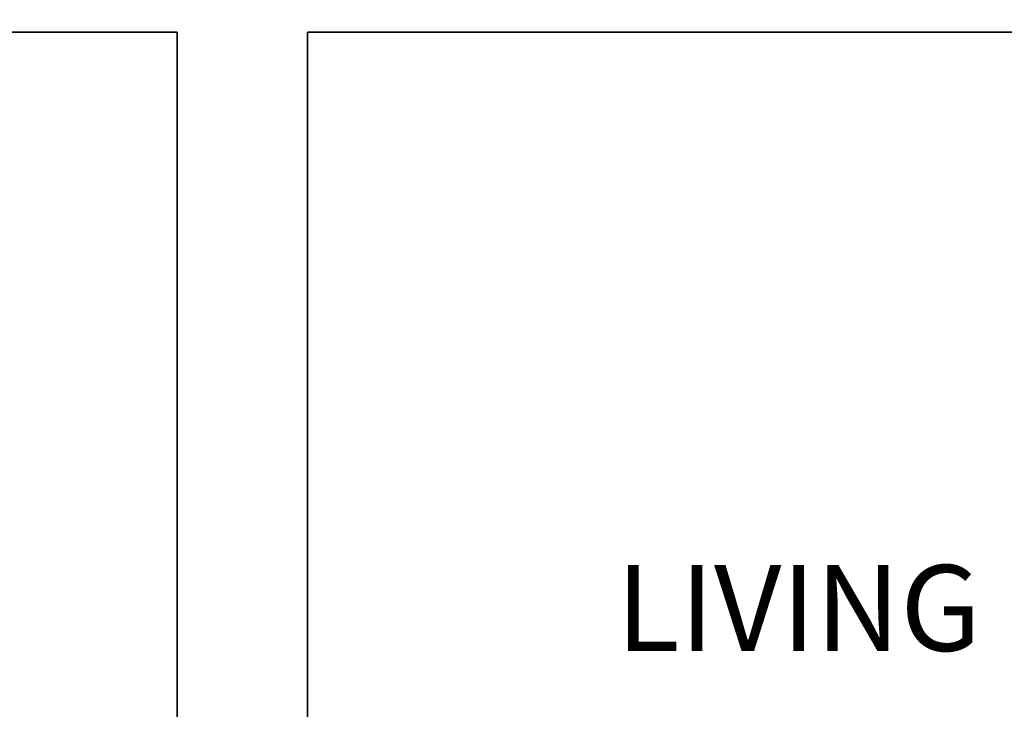
# Model space of a CAD drawing. Units: millimetres. Extents: x 27017497 to 27018854, y 7058029 to 7059154.
# Tile 37 of 91: x 27017621 to 27017689, y 7058386 to 7058433. Entities that reach past the tile are written whole.
import ezdxf

# ---------------------------------------------------------------- set-up
doc = ezdxf.new("R2010")
doc.units = ezdxf.units.MM
for name, color, linetype, lineweight in [('A-ANNO-DIMS', 2, 'Continuous', 18), ('A-AREA-IDEN', 7, 'Continuous', 18), ('A-WALL', 7, 'Continuous', 35)]:
    doc.layers.add(name, color=color, linetype=linetype, lineweight=lineweight)
doc.styles.get("Standard").update_dxf_attribs({"font": 'arial.ttf'})
doc.dimstyles.get("Standard").update_dxf_attribs({"dimtxt": 0.18, "dimasz": 0.18, "dimexe": 0.18, "dimexo": 0.0625, "dimgap": 0.09, "dimtad": 0, "dimtih": 1, "dimtoh": 1, "dimdec": 4, "dimzin": 0, "dimdsep": 46, "dimtxsty": 'Standard', "dimcen": 0.09, "dimadec": 0, "dimazin": 0, "dimtfac": 1, "dimtdec": 4, "dimtofl": 0, "dimtmove": 0, "dimatfit": 3, "dimfxl": 1, "dimtolj": 1, "dimtzin": 0, "dimarcsym": 0})

# ---------------------------------------------------------------- blocks, each defined once
blk = doc.blocks.new('*D48')
at = {"layer": 'A-ANNO-DIMS', "color": 0, "lineweight": -2, "transparency": 16777216}
for p, q in [((27018463.498, 7058622.912), (27017497.536, 7058622.912)), ((27017497.716, 7058622.732), (27017497.716, 7058357.753)), ((27017497.716, 7058092.41), (27017497.716, 7058357.389)), ((27018555.129, 7058092.23), (27017497.536, 7058092.23))]:
    blk.add_line(p, q, dxfattribs=at)
at = {"layer": 'A-ANNO-DIMS', "color": 0, "transparency": 16777216}
for points in [[(27017497.686, 7058622.732), (27017497.746, 7058622.732), (27017497.716, 7058622.912)], [(27017497.686, 7058092.41), (27017497.746, 7058092.41), (27017497.716, 7058092.23)]]:
    blk.add_solid(points, dxfattribs=at)
at = {"layer": 'Defpoints', "color": 0, "transparency": 16777216}
for p in [(27018463.561, 7058622.912), (27017497.716, 7058092.23), (27018555.192, 7058092.23)]:
    blk.add_point(p, dxfattribs=at)
at = {"layer": 'A-ANNO-DIMS', "color": 0, "transparency": 16777216, "insert": (27017497.716, 7058357.571), "char_height": 0.18, "attachment_point": 5}
blk.add_mtext('\\A1;530.7', dxfattribs=at)

msp = doc.modelspace()

# ---------------------------------------------------------------- linework, layer by layer
at = {"layer": 'A-WALL'}
for p, q in [((27017565.666, 7058432.412), (27017632.166, 7058432.412)), ((27017622.666, 7058432.412), (27017632.166, 7058432.412)), ((27017632.166, 7058432.412), (27017632.166, 7058298.912)), ((27017641.166, 7058432.412), (27017641.166, 7058298.912)), ((27017641.166, 7058432.412), (27017716.805, 7058432.412))]:
    msp.add_line(p, q, dxfattribs=at)

# ---------------------------------------------------------------- texts
at = {"layer": 'A-AREA-IDEN'}
msp.add_text('LIVING', height=5.9118, dxfattribs=at).set_placement((27017662.424, 7058389.798))

# ---------------------------------------------------------------- dimensions: what is measured, and where the dimension line sits
at = {"layer": 'A-ANNO-DIMS'}
dim = msp.add_linear_dim(base=(27017497.716, 7058092.23), p1=(27018463.561, 7058622.912), p2=(27018555.192, 7058092.23), angle=90, dimstyle='Standard', override={"dimdec": 1, "dimlfac": 1, "dimrnd": 0, "dimzin": 0, "dimdsep": 46, "dimlunit": 2}, dxfattribs=at)
dim.commit()
dim.dimension.update_dxf_attribs({"geometry": '*D48', "text_midpoint": (27017497.716, 7058357.571)})

doc.saveas('drawing.dxf')
